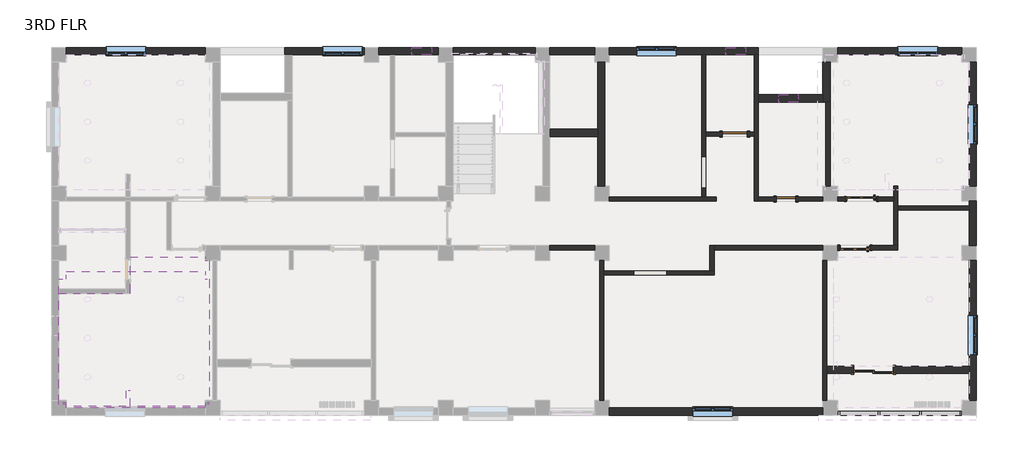
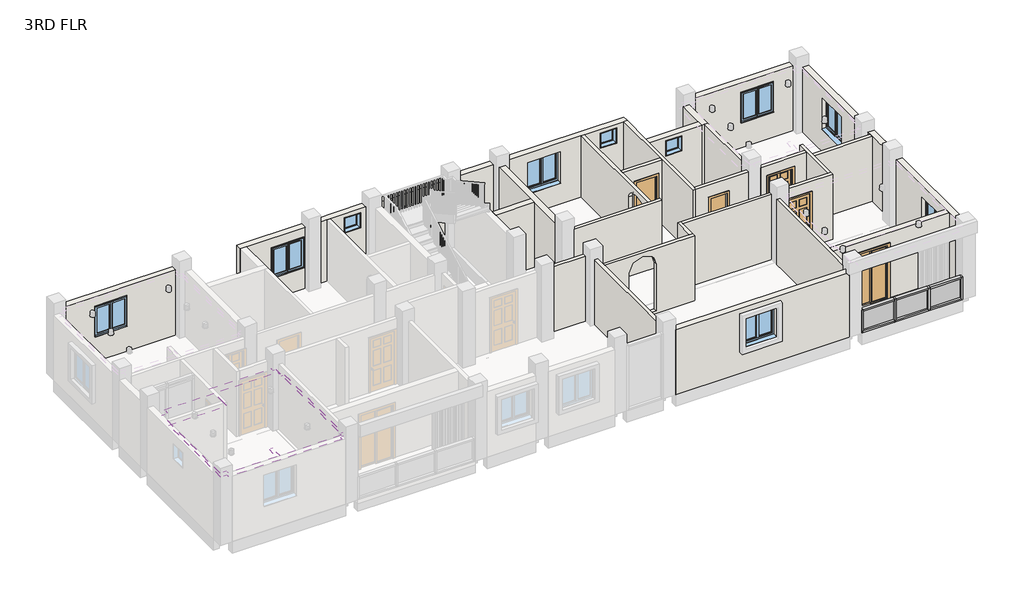
# One storey, part 2 of 5: 32 walls, 10 members, 10 windows, 5 doors, 3 plates, 2 coverings.
"""IFC4 building model written with IfcOpenShell, lengths in millimetres."""

from ifc_helpers import new_model, si_unit, point, frame, frame_2d, origin, place, context, project, spatial, polyline, circle_curve, ellipse_curve, trimmed, segment, composite_curve, outline, extrude, faceted_brep, transform, mapped, element, save
from ifc_brep_helpers import plane_surface, extruded_surface, advanced_brep
from components import door_double_sliding_4436dcad, door_c610b25b, door_03e3dfb5, single_flush_2_x_7_bath_room_door_025d1c86, door_1fe7f57d, member_5d96a33e, member_91edd790, member_410c6227, member_73c23c35, system_panel_glazed_2f542010, system_panel_glazed_876b4d55, window_80340324, w2_0001_4_x_4_window_9dec5fc7

model = new_model("IFC4")

# Units and contexts
model_context = context("Model", 3, world=origin())
ifc_project = project(units=[si_unit("LENGTHUNIT", "METRE", prefix="MILLI")], contexts=[model_context])

# Site, building, storey
site = spatial("IfcSite", under=ifc_project)
building = spatial("IfcBuilding", under=site)
storey = spatial("IfcBuildingStorey", under=building, Name="3RD FLR", Elevation=9448.8)

# Coverings
placement = place(None, origin())
element("IfcCovering", 1, ObjectType="GWB on Mtl. Stud", at=placement, inside=storey, context=model_context, shape_type="SweptSolid", body=[
    extrude(outline(polyline([(-15145.3456086, -10773.5679047), (-15145.3456086, -7363.1659448), (-12959.7401855, -7363.1659448), (-12959.7401855, -6244.0794704), (-10649.5456086, -6244.0794704), (-10649.5456086, -6358.3794704), (-10535.2456086, -6358.3794704), (-10535.2456086, -6963.5679047), (-10535.2456086, -10773.5679047), (-10649.5456086, -10773.5679047), (-10649.5456086, -10887.8679047), (-12959.7401855, -10887.8679047), (-14916.7456086, -10887.8679047), (-14916.7456086, -10773.5679047), (-15145.3456086, -10773.5679047)]), holes=[polyline([(-14840.5456086, -10583.0679047), (-10840.0456086, -10583.0679047), (-10840.0456086, -6548.8794704), (-12654.9401855, -6548.8794704), (-12654.9401855, -7667.9659448), (-14840.5456086, -7667.9659448), (-14840.5456086, -10583.0679047)])]), frame((0.0, 0.0, 11887.2), z_axis=(0.0, 0.0, 1.0), x_axis=(1.0, 0.0, 0.0)), (0.0, 0.0, 1.0), 107.95),
    extrude(outline(polyline([(-14688.1456086, -10430.6679047), (-14688.1456086, -7820.3659448), (-12502.5401855, -7820.3659448), (-12502.5401855, -6701.2794704), (-10992.4456086, -6701.2794704), (-10992.4456086, -10430.6679047), (-14688.1456086, -10430.6679047)]), holes=[polyline([(-14535.7456086, -7972.7659448), (-14535.7456086, -10278.2679047), (-11144.8456086, -10278.2679047), (-11144.8456086, -6853.6794704), (-12350.1401855, -6853.6794704), (-12350.1401855, -7972.7659448), (-14535.7456086, -7972.7659448)])]), frame((0.0, 0.0, 11887.2), z_axis=(0.0, 0.0, 1.0), x_axis=(1.0, 0.0, 0.0)), (0.0, 0.0, 1.0), 107.95),
])
element("IfcCovering", 2, ObjectType="GWB on Mtl. Stud", at=placement, inside=storey, context=model_context, shape_type="SweptSolid", body=[
    extrude(outline(polyline([(-14916.7456086, -6917.1794704), (-14916.7456086, -6688.5794704), (-10649.5456086, -6688.5794704), (-10649.5456086, -6917.1794704), (-10535.2456086, -6917.1794704), (-10535.2456086, -10727.1794704), (-10649.5456086, -10727.1794704), (-10649.5456086, -10841.4794704), (-12959.7401855, -10841.4794704), (-12959.7401855, -10360.3659448), (-13086.7401855, -10360.3659448), (-13086.7401855, -10841.4794704), (-14916.7456086, -10841.4794704), (-14916.7456086, -10727.1794704), (-15145.3456086, -10727.1794704), (-15145.3456086, -6917.1794704), (-14916.7456086, -6917.1794704)]), holes=[composite_curve([segment(trimmed(circle_curve(frame_2d((-14269.0456086, -7552.1794704)), 76.2), [point((-14345.2456086, -7552.1794704))], [point((-14192.8456086, -7552.1794704))], True, "CARTESIAN"), True, "CONTINUOUS"), segment(trimmed(circle_curve(frame_2d((-14269.0456086, -7552.1794704)), 76.2), [point((-14192.8456086, -7552.1794704))], [point((-14345.2456086, -7552.1794704))], True, "CARTESIAN"), True, "CONTINUOUS")], self_intersect=False), composite_curve([segment(trimmed(circle_curve(frame_2d((-14269.0456086, -9939.7794704)), 76.2), [point((-14345.2456086, -9939.7794704))], [point((-14192.8456086, -9939.7794704))], True, "CARTESIAN"), True, "CONTINUOUS"), segment(trimmed(circle_curve(frame_2d((-14269.0456086, -9939.7794704)), 76.2), [point((-14192.8456086, -9939.7794704))], [point((-14345.2456086, -9939.7794704))], True, "CARTESIAN"), True, "CONTINUOUS")], self_intersect=False), composite_curve([segment(trimmed(circle_curve(frame_2d((-14269.0456086, -8745.9794704)), 76.2), [point((-14345.2456086, -8745.9794704))], [point((-14192.8456086, -8745.9794704))], True, "CARTESIAN"), True, "CONTINUOUS"), segment(trimmed(circle_curve(frame_2d((-14269.0456086, -8745.9794704)), 76.2), [point((-14192.8456086, -8745.9794704))], [point((-14345.2456086, -8745.9794704))], True, "CARTESIAN"), True, "CONTINUOUS")], self_intersect=False), composite_curve([segment(trimmed(circle_curve(frame_2d((-11411.5456086, -7552.1794704)), 76.2), [point((-11335.3456086, -7552.1794704))], [point((-11487.7456086, -7552.1794704))], True, "CARTESIAN"), True, "CONTINUOUS"), segment(trimmed(circle_curve(frame_2d((-11411.5456086, -7552.1794704)), 76.2), [point((-11487.7456086, -7552.1794704))], [point((-11335.3456086, -7552.1794704))], True, "CARTESIAN"), True, "CONTINUOUS")], self_intersect=False), composite_curve([segment(trimmed(circle_curve(frame_2d((-11411.5456086, -9939.7794704)), 76.2), [point((-11335.3456086, -9939.7794704))], [point((-11487.7456086, -9939.7794704))], True, "CARTESIAN"), True, "CONTINUOUS"), segment(trimmed(circle_curve(frame_2d((-11411.5456086, -9939.7794704)), 76.2), [point((-11487.7456086, -9939.7794704))], [point((-11335.3456086, -9939.7794704))], True, "CARTESIAN"), True, "CONTINUOUS")], self_intersect=False)]), frame((0.0, 0.0, 12014.2), z_axis=(0.0, 0.0, 1.0), x_axis=(1.0, 0.0, 0.0)), (0.0, 0.0, 1.0), 107.95),
])

# Doors
door_double_sliding_shape = door_double_sliding_4436dcad(model_context)
element("IfcDoor", 3, ObjectType="Door-Double-Sliding", at=placement, inside=storey, context=model_context, shape_type="MappedRepresentation", body=[
    mapped(door_double_sliding_shape, transform((9879.3128058, -9592.4679047, 9448.8), x_axis=(-1.0, 0.0, 0.0), y_axis=(0.0, -1.0, 0.0), z_axis=(0.0, 0.0, 1.0))),
])
door_shape = door_c610b25b(model_context)
element("IfcDoor", 4, ObjectType="Door-Interior-Single-6_Panel-Wood : 36\" x 84\"", at=placement, inside=storey, context=model_context, shape_type="MappedRepresentation", body=[
    mapped(door_shape, transform((9511.0128058, -4462.9044704, 9448.8), x_axis=(-1.0, 0.0, 0.0), y_axis=(0.0, -1.0, 0.0), z_axis=(0.0, 0.0, 1.0))),
])
door_2_shape = door_03e3dfb5(model_context)
element("IfcDoor", 5, ObjectType="Door-Interior-Single-6_Panel-Wood : 36\" x 84\"", at=placement, inside=storey, context=model_context, shape_type="MappedRepresentation", body=[
    mapped(door_2_shape, transform((9307.8128058, -5967.8544704, 9448.8), x_axis=(-1.0, 0.0, 0.0), y_axis=(0.0, -1.0, 0.0), z_axis=(0.0, 0.0, 1.0))),
])
single_flush_2_x_7_bath_room_door_shape = single_flush_2_x_7_bath_room_door_025d1c86(model_context)
element("IfcDoor", 6, ObjectType="Single-Flush : 2' X 7' BATH ROOM DOOR", at=placement, inside=storey, context=model_context, shape_type="MappedRepresentation", body=[
    mapped(single_flush_2_x_7_bath_room_door_shape, transform((7190.4916602, -4466.0794704, 9448.8), x_axis=(1.0, 0.0, 0.0), y_axis=(0.0, 1.0, 0.0), z_axis=(0.0, 0.0, 1.0))),
])
door_3_shape = door_1fe7f57d(model_context)
element("IfcDoor", 7, ObjectType="Single-Flush : 30\" x 80\"", at=placement, inside=storey, context=model_context, shape_type="MappedRepresentation", body=[
    mapped(door_3_shape, transform((5615.6916602, -2472.1794704, 9448.8), x_axis=(1.0, 0.0, 0.0), y_axis=(0.0, 1.0, 0.0), z_axis=(0.0, 0.0, 1.0))),
])

# Members
member_shape = member_5d96a33e(model_context)
element("IfcMember", 8, ObjectType="Rectangular Mullion : 2.5\" x 5\" rectangular", at=placement, inside=storey, context=model_context, shape_type="MappedRepresentation", body=[
    mapped(member_shape, transform((12520.9128058, -11052.9679047, 10363.2), x_axis=(0.0, 0.0, 1.0), y_axis=(0.0, -1.0, 0.0), z_axis=(1.0, 0.0, 0.0))),
])
element("IfcMember", 9, ObjectType="Rectangular Mullion : 2.5\" x 5\" rectangular", at=placement, inside=storey, context=model_context, shape_type="MappedRepresentation", body=[
    mapped(member_shape, transform((10012.6628059, -11052.9679047, 10363.2), x_axis=(0.0, 0.0, 1.0), y_axis=(0.0, -1.0, 0.0), z_axis=(1.0, 0.0, 0.0))),
])
element("IfcMember", 10, ObjectType="Rectangular Mullion : 2.5\" x 5\" rectangular", at=placement, inside=storey, context=model_context, shape_type="MappedRepresentation", body=[
    mapped(member_shape, transform((8837.9128058, -11052.9679047, 9448.8), x_axis=(0.0, 0.0, -1.0), y_axis=(0.0, -1.0, 0.0), z_axis=(-1.0, 0.0, 0.0))),
])
element("IfcMember", 11, ObjectType="Rectangular Mullion : 2.5\" x 5\" rectangular", at=placement, inside=storey, context=model_context, shape_type="MappedRepresentation", body=[
    mapped(member_shape, transform((11346.1628057, -11052.9679047, 9448.8), x_axis=(0.0, 0.0, -1.0), y_axis=(0.0, -1.0, 0.0), z_axis=(-1.0, 0.0, 0.0))),
])
member_2_shape = member_91edd790(model_context)
element("IfcMember", 12, ObjectType="Rectangular Mullion : 2.5\" x 5\" rectangular", at=placement, inside=storey, context=model_context, shape_type="MappedRepresentation", body=[
    mapped(member_2_shape, transform((11282.6628057, -11052.9679047, 10363.2), x_axis=(0.0, 0.0, 1.0), y_axis=(0.0, -1.0, 0.0), z_axis=(1.0, 0.0, 0.0))),
])
element("IfcMember", 13, ObjectType="Rectangular Mullion : 2.5\" x 5\" rectangular", at=placement, inside=storey, context=model_context, shape_type="MappedRepresentation", body=[
    mapped(member_2_shape, transform((10076.1628059, -11052.9679047, 9448.8), x_axis=(0.0, 0.0, -1.0), y_axis=(0.0, -1.0, 0.0), z_axis=(-1.0, 0.0, 0.0))),
])
member_3_shape = member_410c6227(model_context)
element("IfcMember", 14, ObjectType="Rectangular Mullion : 2.5\" x 5\" rectangular", at=placement, inside=storey, context=model_context, shape_type="MappedRepresentation", body=[
    mapped(member_3_shape, transform((10044.4128059, -11052.9679047, 9448.8), x_axis=(1.0, 0.0, 0.0), y_axis=(0.0, -1.0, 0.0), z_axis=(0.0, 0.0, -1.0))),
])
element("IfcMember", 15, ObjectType="Rectangular Mullion : 2.5\" x 5\" rectangular", at=placement, inside=storey, context=model_context, shape_type="MappedRepresentation", body=[
    mapped(member_3_shape, transform((11314.4128057, -11052.9679047, 9448.8), x_axis=(1.0, 0.0, 0.0), y_axis=(0.0, -1.0, 0.0), z_axis=(0.0, 0.0, -1.0))),
])
member_4_shape = member_73c23c35(model_context)
element("IfcMember", 16, ObjectType="Rectangular Mullion : 2.5\" x 5\" rectangular", at=placement, inside=storey, context=model_context, shape_type="MappedRepresentation", body=[
    mapped(member_4_shape, transform((12584.4128058, -11052.9679047, 9448.8), x_axis=(1.0, 0.0, 0.0), y_axis=(0.0, -1.0, 0.0), z_axis=(0.0, 0.0, -1.0))),
])
element("IfcMember", 17, ObjectType="Rectangular Mullion : 2.5\" x 5\" rectangular", at=placement, inside=storey, context=model_context, shape_type="MappedRepresentation", body=[
    mapped(member_4_shape, transform((8774.4128058, -11052.9679047, 10363.2), x_axis=(-1.0, 0.0, 0.0), y_axis=(0.0, -1.0, 0.0), z_axis=(0.0, 0.0, 1.0))),
])

# Plates
system_panel_glazed_shape = system_panel_glazed_2f542010(model_context)
element("IfcPlate", 18, ObjectType="System Panel : Glazed", at=placement, inside=storey, context=model_context, shape_type="MappedRepresentation", body=[
    mapped(system_panel_glazed_shape, transform((9425.2878058, -11052.9679047, 9512.3), x_axis=(1.0, 0.0, 0.0), y_axis=(0.0, 1.0, 0.0), z_axis=(0.0, 0.0, 1.0))),
])
element("IfcPlate", 19, ObjectType="System Panel : Glazed", at=placement, inside=storey, context=model_context, shape_type="MappedRepresentation", body=[
    mapped(system_panel_glazed_shape, transform((11933.5378057, -11052.9679047, 9512.3), x_axis=(1.0, 0.0, 0.0), y_axis=(0.0, 1.0, 0.0), z_axis=(0.0, 0.0, 1.0))),
])
system_panel_glazed_2_shape = system_panel_glazed_876b4d55(model_context)
element("IfcPlate", 20, ObjectType="System Panel : Glazed", at=placement, inside=storey, context=model_context, shape_type="MappedRepresentation", body=[
    mapped(system_panel_glazed_2_shape, transform((10679.4128058, -11052.9679047, 9512.3), x_axis=(1.0, 0.0, 0.0), y_axis=(0.0, 1.0, 0.0), z_axis=(0.0, 0.0, 1.0))),
])

# Walls
element("IfcWall", 21, ObjectType="EXTERIOR WALL 9\"", at=placement, inside=storey, context=model_context, shape_type="SweptSolid", body=[
    extrude(outline(polyline([(9448.8, 1767.5916602), (9448.8, 8317.2128058), (12039.6, 8317.2128058), (12039.6, 1767.5916602), (9448.8, 1767.5916602)]), holes=[polyline([(10448.8, 5552.1916602), (10448.8, 4332.9916602), (11668.0, 4332.9916602), (11668.0, 5552.1916602), (10448.8, 5552.1916602)])]), frame((0.0, -11116.4679047, 0.0), z_axis=(0.0, 1.0, 0.0), x_axis=(0.0, 0.0, 1.0)), (0.0, 0.0, 1.0), 228.6),
])
element("IfcWall", 22, ObjectType="EXTERIOR WALL 9\"", at=placement, inside=storey, context=model_context, shape_type="Brep", body=[
    faceted_brep([(13041.6128058, -10659.2679047, 9448.8), (13041.6128058, -6358.3794704, 9448.8), (13041.6128058, -6358.3794704, 12039.6), (13041.6128058, -10659.2679047, 12039.6), (13041.6128058, -9262.2679047, 10363.2), (13041.6128058, -9262.2679047, 11582.4), (13041.6128058, -8043.0679047, 11582.4), (13041.6128058, -8043.0679047, 10363.2), (12813.0128058, -6358.3794704, 9448.8), (12813.0128058, -9605.1679047, 9448.8), (12813.0128058, -9833.7679047, 9448.8), (12813.0128058, -10659.2679047, 9448.8), (12813.0128058, -10659.2679047, 12039.6), (12813.0128058, -9833.7679047, 12039.6), (12813.0128058, -9605.1679047, 12039.6), (12813.0128058, -6358.3794704, 12039.6), (12813.0128058, -9262.2679047, 11582.4), (12813.0128058, -9262.2679047, 10363.2), (12813.0128058, -8043.0679047, 10363.2), (12813.0128058, -8043.0679047, 11582.4)], [[[0, 1, 2, 3], [4, 5, 6, 7]], [[8, 9, 10, 11, 12, 13, 14, 15], [16, 17, 18, 19]], [[1, 0, 11, 10, 9, 8]], [[2, 1, 8, 15]], [[3, 2, 15, 14, 13, 12]], [[0, 3, 12, 11]], [[5, 4, 17, 16]], [[6, 5, 16, 19]], [[7, 6, 19, 18]], [[4, 7, 18, 17]]]),
])
element("IfcWall", 23, ObjectType="EXTERIOR WALL 9\"", at=placement, inside=storey, context=model_context, shape_type="Brep", body=[
    faceted_brep([(13041.6128058, -5901.1794704, 9448.8), (13041.6128058, -4529.5794704, 9448.8), (13041.6128058, -4529.5794704, 12039.6), (13041.6128058, -5901.1794704, 12039.6), (12813.0128058, -5901.1794704, 9448.8), (12813.0128058, -5901.1794704, 12039.6), (12813.0128058, -4808.9794704, 12039.6), (12813.0128058, -4681.9794704, 12039.6), (12813.0128058, -4529.5794704, 12039.6), (12813.0128058, -4529.5794704, 9448.8), (12813.0128058, -4681.9794704, 9448.8), (12813.0128058, -4808.9794704, 9448.8)], [[[0, 1, 2, 3]], [[4, 5, 6, 7, 8, 9, 10, 11]], [[1, 0, 4, 11, 10, 9]], [[2, 1, 9, 8]], [[3, 2, 8, 7, 6, 5]], [[0, 3, 5, 4]]]),
])
element("IfcWall", 24, ObjectType="EXTERIOR WALL 9\"", at=placement, inside=storey, context=model_context, shape_type="SweptSolid", body=[
    extrude(outline(polyline([(-4072.3794704, 9448.8), (-4072.3794704, 12039.6), (-262.3794704, 12039.6), (-262.3794704, 9448.8), (-4072.3794704, 9448.8)]), holes=[polyline([(-2776.9794704, 10363.2), (-1557.7794704, 10363.2), (-1557.7794704, 11582.4), (-2776.9794704, 11582.4), (-2776.9794704, 10363.2)])]), frame((12813.0128058, 0.0, 0.0), z_axis=(1.0, 0.0, 0.0), x_axis=(0.0, 1.0, 0.0)), (0.0, 0.0, 1.0), 228.6),
])
element("IfcWall", 25, ObjectType="EXTERIOR WALL 9\"", at=placement, inside=storey, context=model_context, shape_type="SweptSolid", body=[
    extrude(outline(polyline([(9448.8, 12584.4128058), (12039.6, 12584.4128058), (12039.6, 8774.4128058), (9448.8, 8774.4128058), (9448.8, 12584.4128058)]), holes=[polyline([(10448.8, 10628.6128058), (11668.0, 10628.6128058), (11668.0, 11847.8128058), (10448.8, 11847.8128058), (10448.8, 10628.6128058)])]), frame((0.0, -33.7794704, 0.0), z_axis=(0.0, 1.0, 0.0), x_axis=(0.0, 0.0, 1.0)), (0.0, 0.0, 1.0), 228.6),
])
element("IfcWall", 26, ObjectType="EXTERIOR WALL 9\"", at=placement, inside=storey, context=model_context, shape_type="SweptSolid", body=[
    extrude(outline(polyline([(9448.8, -14916.7456086), (9448.8, -10649.5456086), (12039.6, -10649.5456086), (12039.6, -14916.7456086), (9448.8, -14916.7456086)]), holes=[polyline([(10448.8, -13697.5456086), (11668.0, -13697.5456086), (11668.0, -12478.3456086), (10448.8, -12478.3456086), (10448.8, -13697.5456086)])]), frame((0.0, -33.7794704, 0.0), z_axis=(0.0, 1.0, 0.0), x_axis=(0.0, 0.0, 1.0)), (0.0, 0.0, 1.0), 228.6),
])
element("IfcWall", 27, ObjectType="EXTERIOR WALL 9\"", at=placement, inside=storey, context=model_context, shape_type="SweptSolid", body=[
    extrude(outline(polyline([(9448.8, 8444.2128058), (9448.8, 9269.7128058), (11582.4, 9269.7128058), (11582.4, 10488.9128058), (9448.8, 10488.9128058), (9448.8, 12813.0128058), (12039.6, 12813.0128058), (12039.6, 8444.2128058), (9448.8, 8444.2128058)])), frame((0.0, -9833.7679047, 0.0), z_axis=(0.0, 1.0, 0.0), x_axis=(0.0, 0.0, 1.0)), (0.0, 0.0, 1.0), 228.6),
])
element("IfcWall", 28, ObjectType="EXTERIOR WALL 9\"", at=placement, inside=storey, context=model_context, shape_type="Brep", body=[
    faceted_brep([(-5772.7456086, 194.8205296, 9448.8), (-8211.1456086, 194.8205296, 9448.8), (-8211.1456086, 194.8205296, 12039.6), (-5772.7456086, 194.8205296, 12039.6), (-7042.7456086, 194.8205296, 10448.8), (-5823.5456086, 194.8205296, 10448.8), (-5823.5456086, 194.8205296, 11668.0), (-7042.7456086, 194.8205296, 11668.0), (-5772.7456086, -33.7794704, 9448.8), (-5772.7456086, -33.7794704, 12039.6), (-7982.5456086, -33.7794704, 12039.6), (-8211.1456086, -33.7794704, 12039.6), (-8211.1456086, -33.7794704, 9448.8), (-7982.5456086, -33.7794704, 9448.8), (-7042.7456086, -33.7794704, 10448.8), (-7042.7456086, -33.7794704, 11668.0), (-5823.5456086, -33.7794704, 11668.0), (-5823.5456086, -33.7794704, 10448.8)], [[[0, 1, 2, 3], [4, 5, 6, 7]], [[8, 9, 10, 11, 12, 13], [14, 15, 16, 17]], [[1, 0, 8, 13, 12]], [[3, 2, 11, 10, 9]], [[0, 3, 9, 8]], [[2, 1, 12, 11]], [[15, 14, 4, 7]], [[16, 15, 7, 6]], [[17, 16, 6, 5]], [[14, 17, 5, 4]]]),
])
element("IfcWall", 29, ObjectType="EXTERIOR WALL 9\"", at=placement, inside=storey, context=model_context, shape_type="Brep", body=[
    faceted_brep([(-5315.5456086, -33.7794704, 9448.8), (-4959.9456086, -33.7794704, 9448.8), (-4832.9456086, -33.7794704, 9448.8), (-3486.7456086, -33.7794704, 9448.8), (-3486.7456086, -33.7794704, 12039.6), (-4832.9456086, -33.7794704, 12039.6), (-4959.9456086, -33.7794704, 12039.6), (-5315.5456086, -33.7794704, 12039.6), (-3689.9456086, -33.7794704, 11887.2), (-3689.9456086, -33.7794704, 11277.6), (-4299.5456086, -33.7794704, 11277.6), (-4299.5456086, -33.7794704, 11887.2), (-3486.7456086, 194.8205296, 9448.8), (-5315.5456086, 194.8205296, 9448.8), (-5315.5456086, 194.8205296, 12039.6), (-3486.7456086, 194.8205296, 12039.6), (-3689.9456086, 194.8205296, 11277.6), (-3689.9456086, 194.8205296, 11887.2), (-4299.5456086, 194.8205296, 11887.2), (-4299.5456086, 194.8205296, 11277.6)], [[[0, 1, 2, 3, 4, 5, 6, 7], [8, 9, 10, 11]], [[12, 13, 14, 15], [16, 17, 18, 19]], [[3, 2, 1, 0, 13, 12]], [[4, 3, 12, 15]], [[7, 6, 5, 4, 15, 14]], [[0, 7, 14, 13]], [[8, 17, 16, 9]], [[9, 16, 19, 10]], [[10, 19, 18, 11]], [[17, 8, 11, 18]]]),
])
element("IfcWall", 30, ObjectType="EXTERIOR WALL 9\"", at=placement, inside=storey, context=model_context, shape_type="SweptSolid", body=[
    extrude(outline(polyline([(-518.4083398, -33.7794704), (-3029.5456086, -33.7794704), (-3029.5456086, 194.8205296), (-518.4083398, 194.8205296), (-518.4083398, -33.7794704)])), frame((0.0, 0.0, 9448.8), z_axis=(0.0, 0.0, 1.0), x_axis=(1.0, 0.0, 0.0)), (0.0, 0.0, 1.0), 2590.8),
])
element("IfcWall", 31, ObjectType="EXTERIOR WALL 9\"", at=placement, inside=storey, context=model_context, shape_type="SweptSolid", body=[
    extrude(outline(polyline([(1310.3916602, -33.7794704), (-61.2083398, -33.7794704), (-61.2083398, 194.8205296), (1310.3916602, 194.8205296), (1310.3916602, -33.7794704)])), frame((0.0, 0.0, 9448.8), z_axis=(0.0, 0.0, 1.0), x_axis=(1.0, 0.0, 0.0)), (0.0, 0.0, 1.0), 2590.8),
])
element("IfcWall", 32, ObjectType="EXTERIOR WALL 9\"", at=placement, inside=storey, context=model_context, shape_type="Brep", body=[
    faceted_brep([(1767.5916602, -33.7794704, 9448.8), (4599.6916602, -33.7794704, 9448.8), (4726.6916602, -33.7794704, 9448.8), (6212.5916602, -33.7794704, 9448.8), (6339.5916602, -33.7794704, 9448.8), (6339.5916602, -33.7794704, 12039.6), (6212.5916602, -33.7794704, 12039.6), (4726.6916602, -33.7794704, 12039.6), (4599.6916602, -33.7794704, 12039.6), (1767.5916602, -33.7794704, 12039.6), (3824.9916602, -33.7794704, 11668.0), (3824.9916602, -33.7794704, 10448.8), (2605.7916602, -33.7794704, 10448.8), (2605.7916602, -33.7794704, 11668.0), (5945.8916602, -33.7794704, 11887.2), (5945.8916602, -33.7794704, 11277.6), (5336.2916602, -33.7794704, 11277.6), (5336.2916602, -33.7794704, 11887.2), (6339.5916602, 194.8205296, 9448.8), (1767.5916602, 194.8205296, 9448.8), (1767.5916602, 194.8205296, 12039.6), (6339.5916602, 194.8205296, 12039.6), (3824.9916602, 194.8205296, 10448.8), (3824.9916602, 194.8205296, 11668.0), (2605.7916602, 194.8205296, 11668.0), (2605.7916602, 194.8205296, 10448.8), (5945.8916602, 194.8205296, 11277.6), (5945.8916602, 194.8205296, 11887.2), (5336.2916602, 194.8205296, 11887.2), (5336.2916602, 194.8205296, 11277.6)], [[[0, 1, 2, 3, 4, 5, 6, 7, 8, 9], [10, 11, 12, 13], [14, 15, 16, 17]], [[18, 19, 20, 21], [22, 23, 24, 25], [26, 27, 28, 29]], [[4, 3, 2, 1, 0, 19, 18]], [[9, 8, 7, 6, 5, 21, 20]], [[0, 9, 20, 19]], [[5, 4, 18, 21]], [[23, 22, 11, 10]], [[24, 23, 10, 13]], [[25, 24, 13, 12]], [[22, 25, 12, 11]], [[14, 27, 26, 15]], [[15, 26, 29, 16]], [[16, 29, 28, 17]], [[27, 14, 17, 28]]]),
])
element("IfcWall", 33, ObjectType="EXTERIOR WALL 9\"", at=placement, inside=storey, context=model_context, shape_type="Brep", body=[
    faceted_brep([(8317.2128058, -262.3794704, 9448.8), (8317.2128058, -1252.9794704, 9448.8), (8317.2128058, -1481.5794704, 9448.8), (8317.2128058, -1481.5794704, 12039.6), (8317.2128058, -1252.9794704, 12039.6), (8317.2128058, -262.3794704, 12039.6), (8545.8128058, -262.3794704, 9448.8), (8545.8128058, -262.3794704, 12039.6), (8545.8128058, -1481.5794704, 12039.6), (8545.8128058, -1481.5794704, 9448.8), (8418.8128058, -1481.5794704, 9448.8), (8418.8128058, -1481.5794704, 12039.6)], [[[0, 1, 2, 3, 4, 5]], [[6, 7, 8, 9]], [[2, 1, 0, 6, 9, 10]], [[5, 4, 3, 11, 8, 7]], [[0, 5, 7, 6]], [[3, 2, 10, 9, 8, 11]]]),
])
element("IfcWall", 34, ObjectType="EXTERIOR WALL 9\"", at=placement, inside=storey, context=model_context, shape_type="SweptSolid", body=[
    extrude(outline(polyline([(9448.8, 6339.5916602), (9448.8, 8317.2128058), (12039.6, 8317.2128058), (12039.6, 6339.5916602), (9448.8, 6339.5916602)]), holes=[polyline([(11887.2, 7571.4916602), (11277.6, 7571.4916602), (11277.6, 6961.8916602), (11887.2, 6961.8916602), (11887.2, 7571.4916602)])]), frame((0.0, -1481.5794704, 0.0), z_axis=(0.0, 1.0, 0.0), x_axis=(0.0, 0.0, 1.0)), (0.0, 0.0, 1.0), 228.6),
])
element("IfcWall", 35, ObjectType="EXTERIOR WALL 9\"", at=placement, inside=storey, context=model_context, shape_type="Brep", body=[
    faceted_brep([(1399.2916602, -262.3794704, 9448.8), (1399.2916602, -2319.7794704, 9448.8), (1399.2916602, -2548.3794704, 9448.8), (1399.2916602, -4072.3794704, 9448.8), (1399.2916602, -4072.3794704, 12039.6), (1399.2916602, -2548.3794704, 12039.6), (1399.2916602, -2319.7794704, 12039.6), (1399.2916602, -262.3794704, 12039.6), (1627.8916602, -262.3794704, 9448.8), (1627.8916602, -262.3794704, 12039.6), (1627.8916602, -4072.3794704, 12039.6), (1627.8916602, -4072.3794704, 9448.8)], [[[0, 1, 2, 3, 4, 5, 6, 7]], [[8, 9, 10, 11]], [[3, 2, 1, 0, 8, 11]], [[4, 3, 11, 10]], [[7, 6, 5, 4, 10, 9]], [[0, 7, 9, 8]]]),
])
element("IfcWall", 36, ObjectType="EXTERIOR WALL 9\"", at=placement, inside=storey, context=model_context, shape_type="SweptSolid", body=[
    extrude(outline(polyline([(1399.2916602, -2548.3794704), (-61.2083398, -2548.3794704), (-61.2083398, -2319.7794704), (1399.2916602, -2319.7794704), (1399.2916602, -2548.3794704)])), frame((0.0, 0.0, 9448.8), z_axis=(0.0, 0.0, 1.0), x_axis=(1.0, 0.0, 0.0)), (0.0, 0.0, 1.0), 2590.8),
])
element("IfcWall", 37, ObjectType="INTERIOR WALL 5\"", at=placement, inside=storey, context=model_context, shape_type="Brep", body=[
    faceted_brep([(1589.7916602, -10659.2679047, 9448.8), (1589.7916602, -6802.8794704, 9448.8), (1589.7916602, -6675.8794704, 9448.8), (1589.7916602, -6358.3794704, 9448.8), (1589.7916602, -6358.3794704, 12039.6), (1589.7916602, -6675.8794704, 12039.6), (1589.7916602, -6802.8794704, 12039.6), (1589.7916602, -10659.2679047, 12039.6), (1462.7916602, -10659.2679047, 9448.8), (1462.7916602, -10659.2679047, 12039.6), (1462.7916602, -6358.3794704, 12039.6), (1462.7916602, -6358.3794704, 9448.8)], [[[0, 1, 2, 3, 4, 5, 6, 7]], [[8, 9, 10, 11]], [[3, 2, 1, 0, 8, 11]], [[4, 3, 11, 10]], [[7, 6, 5, 4, 10, 9]], [[0, 7, 9, 8]]]),
])
element("IfcWall", 38, ObjectType="INTERIOR WALL 5\"", at=placement, inside=storey, context=model_context, shape_type="Brep", body=[
    faceted_brep([(8444.2128058, -10659.2679047, 9448.8), (8444.2128058, -9833.7679047, 9448.8), (8444.2128058, -9605.1679047, 9448.8), (8444.2128058, -6358.3794704, 9448.8), (8444.2128058, -6358.3794704, 12039.6), (8444.2128058, -9605.1679047, 12039.6), (8444.2128058, -9833.7679047, 12039.6), (8444.2128058, -10659.2679047, 12039.6), (8317.2128058, -10659.2679047, 9448.8), (8317.2128058, -10659.2679047, 12039.6), (8317.2128058, -6358.3794704, 12039.6), (8317.2128058, -6358.3794704, 9448.8)], [[[0, 1, 2, 3, 4, 5, 6, 7]], [[8, 9, 10, 11]], [[3, 2, 1, 0, 8, 11]], [[4, 3, 11, 10]], [[7, 6, 5, 4, 10, 9]], [[0, 7, 9, 8]]]),
])
element("IfcWall", 39, ObjectType="INTERIOR WALL 5\"", at=placement, inside=storey, context=model_context, shape_type="SweptSolid", body=[
    extrude(outline(polyline([(10628.6128058, -4681.9794704), (12813.0128058, -4681.9794704), (12813.0128058, -4808.9794704), (10628.6128058, -4808.9794704), (10628.6128058, -4681.9794704)])), frame((0.0, 0.0, 9448.8), z_axis=(0.0, 0.0, 1.0), x_axis=(1.0, 0.0, 0.0)), (0.0, 0.0, 1.0), 2590.8),
])
element("IfcWall", 40, ObjectType="INTERIOR WALL 5\"", at=placement, inside=storey, context=model_context, shape_type="Brep", body=[
    faceted_brep([(10628.6128058, -6028.1794704, 12039.6), (8774.4128058, -6028.1794704, 12039.6), (8774.4128058, -6028.1794704, 9448.8), (8825.2128058, -6028.1794704, 9448.8), (8825.2128058, -6028.1794704, 11607.8), (9790.4128058, -6028.1794704, 11607.8), (9790.4128058, -6028.1794704, 9448.8), (10628.6128058, -6028.1794704, 9448.8), (8774.4128058, -5901.1794704, 12039.6), (10501.6128058, -5901.1794704, 12039.6), (10628.6128058, -5901.1794704, 12039.6), (10628.6128058, -5901.1794704, 9448.8), (10501.6128058, -5901.1794704, 9448.8), (9790.4128058, -5901.1794704, 9448.8), (9790.4128058, -5901.1794704, 11607.8), (8825.2128058, -5901.1794704, 11607.8), (8825.2128058, -5901.1794704, 9448.8), (8774.4128058, -5901.1794704, 9448.8)], [[[0, 1, 2, 3, 4, 5, 6, 7]], [[8, 9, 10, 11, 12, 13, 14, 15, 16, 17]], [[2, 17, 16, 3]], [[11, 7, 6, 13, 12]], [[1, 0, 10, 9, 8]], [[2, 1, 8, 17]], [[0, 7, 11, 10]], [[15, 4, 3, 16]], [[4, 15, 14, 5]], [[5, 14, 13, 6]]]),
])
element("IfcWall", 41, ObjectType="INTERIOR WALL 5\"", at=placement, inside=storey, context=model_context, shape_type="Brep", body=[
    faceted_brep([(10628.6128058, -5901.1794704, 9448.8), (10628.6128058, -4808.9794704, 9448.8), (10628.6128058, -4681.9794704, 9448.8), (10628.6128058, -4072.3794704, 9448.8), (10628.6128058, -4072.3794704, 12039.6), (10628.6128058, -4681.9794704, 12039.6), (10628.6128058, -4808.9794704, 12039.6), (10628.6128058, -5901.1794704, 12039.6), (10501.6128058, -5901.1794704, 9448.8), (10501.6128058, -5901.1794704, 12039.6), (10501.6128058, -4529.5794704, 12039.6), (10501.6128058, -4402.5794704, 12039.6), (10501.6128058, -4072.3794704, 12039.6), (10501.6128058, -4072.3794704, 9448.8), (10501.6128058, -4402.5794704, 9448.8), (10501.6128058, -4529.5794704, 9448.8)], [[[0, 1, 2, 3, 4, 5, 6, 7]], [[8, 9, 10, 11, 12, 13, 14, 15]], [[3, 2, 1, 0, 8, 15, 14, 13]], [[4, 3, 13, 12]], [[7, 6, 5, 4, 12, 11, 10, 9]], [[0, 7, 9, 8]]]),
])
element("IfcWall", 42, ObjectType="INTERIOR WALL 5\"", at=placement, inside=storey, context=model_context, shape_type="Brep", body=[
    faceted_brep([(6212.5916602, -33.7794704, 9448.8), (6212.5916602, -2408.6794704, 9448.8), (6212.5916602, -2535.6794704, 9448.8), (6212.5916602, -4529.5794704, 9448.8), (6212.5916602, -4529.5794704, 12039.6), (6212.5916602, -2535.6794704, 12039.6), (6212.5916602, -2408.6794704, 12039.6), (6212.5916602, -33.7794704, 12039.6), (6339.5916602, -33.7794704, 9448.8), (6339.5916602, -33.7794704, 12039.6), (6339.5916602, -1252.9794704, 12039.6), (6339.5916602, -1481.5794704, 12039.6), (6339.5916602, -4402.5794704, 12039.6), (6339.5916602, -4529.5794704, 12039.6), (6339.5916602, -4529.5794704, 9448.8), (6339.5916602, -4402.5794704, 9448.8), (6339.5916602, -1481.5794704, 9448.8), (6339.5916602, -1252.9794704, 9448.8)], [[[0, 1, 2, 3, 4, 5, 6, 7]], [[8, 9, 10, 11, 12, 13, 14, 15, 16, 17]], [[3, 2, 1, 0, 8, 17, 16, 15, 14]], [[7, 6, 5, 4, 13, 12, 11, 10, 9]], [[0, 7, 9, 8]], [[4, 3, 14, 13]]]),
])
element("IfcWall", 43, ObjectType="INTERIOR WALL 5\"", at=placement, inside=storey, context=model_context, shape_type="SweptSolid", body=[
    extrude(outline(polyline([(8418.8128058, -4072.3794704), (8418.8128058, -1481.5794704), (8545.8128058, -1481.5794704), (8545.8128058, -4072.3794704), (8418.8128058, -4072.3794704)])), frame((0.0, 0.0, 9448.8), z_axis=(0.0, 0.0, 1.0), x_axis=(1.0, 0.0, 0.0)), (0.0, 0.0, 1.0), 2590.8),
])
element("IfcWall", 44, ObjectType="INTERIOR WALL 5\"", at=placement, inside=storey, context=model_context, shape_type="Brep", body=[
    faceted_brep([(1767.5916602, -4529.5794704, 9448.8), (5044.1916602, -4529.5794704, 9448.8), (5044.1916602, -4529.5794704, 12039.6), (1767.5916602, -4529.5794704, 12039.6), (1767.5916602, -4402.5794704, 9448.8), (1767.5916602, -4402.5794704, 12039.6), (4599.6916602, -4402.5794704, 12039.6), (4726.6916602, -4402.5794704, 12039.6), (5044.1916602, -4402.5794704, 12039.6), (5044.1916602, -4402.5794704, 9448.8), (4726.6916602, -4402.5794704, 9448.8), (4599.6916602, -4402.5794704, 9448.8)], [[[0, 1, 2, 3]], [[4, 5, 6, 7, 8, 9, 10, 11]], [[1, 0, 4, 11, 10, 9]], [[2, 1, 9, 8]], [[3, 2, 8, 7, 6, 5]], [[0, 3, 5, 4]]]),
])
element("IfcWall", 45, ObjectType="INTERIOR WALL 5\"", at=placement, inside=storey, context=model_context, shape_type="AdvancedBrep", body=[
    advanced_brep(
    [(4599.6916602, -33.7794704, 9448.8), (4599.6916602, -4402.5794704, 9448.8), (4599.6916602, -4402.5794704, 12039.6), (4599.6916602, -33.7794704, 12039.6), (4599.6916602, -3162.9760679, 11507.4701015), (4599.6916602, -4128.1760679, 11507.4701015), (4599.6916602, -4128.1760679, 9627.8701015), (4599.6916602, -3162.9760679, 9627.8701015), (4726.6916602, -33.7794704, 9448.8), (4726.6916602, -33.7794704, 12039.6), (4726.6916602, -2408.6794704, 12039.6), (4726.6916602, -2535.6794704, 12039.6), (4726.6916602, -4402.5794704, 12039.6), (4726.6916602, -4402.5794704, 9448.8), (4726.6916602, -2535.6794704, 9448.8), (4726.6916602, -2408.6794704, 9448.8), (4726.6916602, -3162.9760679, 11507.4701015), (4726.6916602, -3162.9760679, 9627.8701015), (4726.6916602, -4128.1760679, 9627.8701015), (4726.6916602, -4128.1760679, 11507.4701015)],
    [
        (0, 1),
        (1, 2),
        (2, 3),
        (3, 0),
        (4, 5, ellipse_curve(frame((4599.6916602, -3645.5760679, 11507.4701015), z_axis=(1.0, 0.0, 0.0), x_axis=(0.0, -1.0, 0.0)), 482.6, 330.2)),
        (5, 6),
        (6, 7),
        (7, 4),
        (8, 9),
        (9, 10),
        (10, 11),
        (11, 12),
        (12, 13),
        (13, 14),
        (14, 15),
        (15, 8),
        (16, 17),
        (17, 18),
        (18, 19),
        (19, 16, ellipse_curve(frame((4726.6916602, -3645.5760679, 11507.4701015), z_axis=(-1.0, 0.0, 0.0), x_axis=(0.0, -1.0, 0.0)), 482.6, 330.2)),
        (3, 9),
        (8, 0),
        (1, 13),
        (12, 2),
        (4, 16),
        (19, 5),
        (18, 6),
        (17, 7),
    ],
    [
        plane_surface(frame((4599.6916602, 80.5205296, 9448.8), z_axis=(-1.0, 0.0, 0.0), x_axis=(0.0, -1.0, 0.0))),
        plane_surface(frame((4726.6916602, 80.5205296, 9448.8), z_axis=(1.0, 0.0, 0.0), x_axis=(0.0, 1.0, 0.0))),
        plane_surface(frame((1784.6412895, -33.7794704, 9448.8), z_axis=(0.0, 1.0, 0.0), x_axis=(1.0, 0.0, 0.0))),
        plane_surface(frame((1767.5916602, -4402.5794704, 9448.8), z_axis=(0.0, -1.0, 0.0), x_axis=(-1.0, 0.0, 0.0))),
        plane_surface(frame((4599.6916602, 80.5205296, 9448.8), z_axis=(0.0, 0.0, -1.0), x_axis=(1.0, 0.0, 0.0))),
        plane_surface(frame((4599.6916602, -4466.0794704, 12039.6), z_axis=(0.0, 0.0, 1.0), x_axis=(1.0, 0.0, 0.0))),
        extruded_surface(trimmed(ellipse_curve(frame((4790.1916602, -3645.5760679, 11507.4701015), z_axis=(1.0, 0.0, 0.0), x_axis=(0.0, -1.0, 0.0)), 482.6, 330.2), [point((4790.1916602, -3162.9760679, 11507.4701015))], [point((4790.1916602, -4128.1760679, 11507.4701015))], True, "CARTESIAN"), (-127.0, 0.0, 0.0), 127.0),
        plane_surface(frame((4599.6916602, -4128.1760679, 11507.4701015), z_axis=(0.0, 1.0, 0.0), x_axis=(1.0, 0.0, 0.0))),
        plane_surface(frame((4599.6916602, -4128.1760679, 9627.8701015), z_axis=(0.0, 0.0, 1.0), x_axis=(1.0, 0.0, 0.0))),
        plane_surface(frame((4599.6916602, -3162.9760679, 9627.8701015), z_axis=(0.0, -1.0, 0.0), x_axis=(1.0, 0.0, 0.0))),
    ],
    [
        (0, [[1, 2, 3, 4], [5, 6, 7, 8]]),
        (1, [[9, 10, 11, 12, 13, 14, 15, 16], [17, 18, 19, 20]]),
        (2, [[-4, 21, -9, 22]]),
        (3, [[-2, 23, -13, 24]]),
        (4, [[-1, -22, -16, -15, -14, -23]]),
        (5, [[-3, -24, -12, -11, -10, -21]]),
        (6, [[-5, 25, -20, 26]]),
        (7, [[-6, -26, -19, 27]]),
        (8, [[-7, -27, -18, 28]]),
        (9, [[-8, -28, -17, -25]]),
    ],
),
])
element("IfcWall", 46, ObjectType="INTERIOR WALL 5\"", at=placement, inside=storey, context=model_context, shape_type="SweptSolid", body=[
    extrude(outline(polyline([(11480.8, 5996.6916602), (9448.8, 5996.6916602), (9448.8, 6212.5916602), (12039.6, 6212.5916602), (12039.6, 4726.6916602), (9448.8, 4726.6916602), (9448.8, 5234.6916602), (11480.8, 5234.6916602), (11480.8, 5996.6916602)])), frame((0.0, -2535.6794704, 0.0), z_axis=(0.0, 1.0, 0.0), x_axis=(0.0, 0.0, 1.0)), (0.0, 0.0, 1.0), 127.0),
])
element("IfcWall", 47, ObjectType="INTERIOR WALL 5\"", at=placement, inside=storey, context=model_context, shape_type="SweptSolid", body=[
    extrude(outline(polyline([(11480.8, 7495.2916602), (9448.8, 7495.2916602), (9448.8, 8317.2128058), (12039.6, 8317.2128058), (12039.6, 6339.5916602), (9448.8, 6339.5916602), (9448.8, 6885.6916602), (11480.8, 6885.6916602), (11480.8, 7495.2916602)])), frame((0.0, -4529.5794704, 0.0), z_axis=(0.0, 1.0, 0.0), x_axis=(0.0, 0.0, 1.0)), (0.0, 0.0, 1.0), 127.0),
])
element("IfcWall", 48, ObjectType="INTERIOR WALL 5\"", at=placement, inside=storey, context=model_context, shape_type="SweptSolid", body=[
    extrude(outline(polyline([(12039.6, 10501.6128058), (12039.6, 8774.4128058), (9448.8, 8774.4128058), (9448.8, 9028.4128058), (11607.8, 9028.4128058), (11607.8, 9993.6128058), (9448.8, 9993.6128058), (9448.8, 10501.6128058), (12039.6, 10501.6128058)])), frame((0.0, -4529.5794704, 0.0), z_axis=(0.0, 1.0, 0.0), x_axis=(0.0, 0.0, 1.0)), (0.0, 0.0, 1.0), 127.0),
])
element("IfcWall", 49, ObjectType="INTERIOR WALL 5\"", at=placement, inside=storey, context=model_context, shape_type="SweptSolid", body=[
    extrude(outline(polyline([(-61.2083398, -5901.1794704), (1310.3916602, -5901.1794704), (1310.3916602, -6028.1794704), (-61.2083398, -6028.1794704), (-61.2083398, -5901.1794704)])), frame((0.0, 0.0, 9448.8), z_axis=(0.0, 0.0, 1.0), x_axis=(1.0, 0.0, 0.0)), (0.0, 0.0, 1.0), 2590.8),
])
element("IfcWall", 50, ObjectType="INTERIOR WALL 5\"", at=placement, inside=storey, context=model_context, shape_type="AdvancedBrep", body=[
    advanced_brep(
    [(1589.7916602, -6802.8794704, 9448.8), (4980.6916602, -6802.8794704, 9448.8), (4980.6916602, -6802.8794704, 12039.6), (1589.7916602, -6802.8794704, 12039.6), (2514.6258025, -6802.8794704, 11411.5597277), (3530.6258025, -6802.8794704, 11411.5597277), (3530.6258025, -6802.8794704, 9557.3597277), (2514.6258025, -6802.8794704, 9557.3597277), (1589.7916602, -6675.8794704, 9448.8), (1589.7916602, -6675.8794704, 12039.6), (4853.6916602, -6675.8794704, 12039.6), (4980.6916602, -6675.8794704, 12039.6), (4980.6916602, -6675.8794704, 9448.8), (4853.6916602, -6675.8794704, 9448.8), (2514.6258025, -6675.8794704, 11411.5597277), (2514.6258025, -6675.8794704, 9557.3597277), (3530.6258025, -6675.8794704, 9557.3597277), (3530.6258025, -6675.8794704, 11411.5597277)],
    [
        (0, 1),
        (1, 2),
        (2, 3),
        (3, 0),
        (4, 5, ellipse_curve(frame((3022.6258025, -6802.8794704, 11411.5597277), z_axis=(0.0, 1.0, 0.0), x_axis=(-1.0, 0.0, 0.0)), 508.0, 482.6)),
        (5, 6),
        (6, 7),
        (7, 4),
        (8, 9),
        (9, 10),
        (10, 11),
        (11, 12),
        (12, 13),
        (13, 8),
        (14, 15),
        (15, 16),
        (16, 17),
        (17, 14, ellipse_curve(frame((3022.6258025, -6675.8794704, 11411.5597277), z_axis=(0.0, -1.0, 0.0), x_axis=(-1.0, 0.0, 0.0)), 508.0, 482.6)),
        (3, 9),
        (8, 0),
        (1, 12),
        (11, 2),
        (4, 14),
        (17, 5),
        (16, 6),
        (15, 7),
    ],
    [
        plane_surface(frame((1526.2916602, -6802.8794704, 9448.8), z_axis=(0.0, -1.0, 0.0), x_axis=(1.0, 0.0, 0.0))),
        plane_surface(frame((1526.2916602, -6675.8794704, 9448.8), z_axis=(0.0, 1.0, 0.0), x_axis=(-1.0, 0.0, 0.0))),
        plane_surface(frame((1589.7916602, -10648.7570633, 9448.8), z_axis=(-1.0, 0.0, 0.0), x_axis=(0.0, 1.0, 0.0))),
        plane_surface(frame((4980.6916602, -6675.8794704, 9448.8), z_axis=(1.0, 0.0, 0.0), x_axis=(0.0, 1.0, 0.0))),
        plane_surface(frame((1526.2916602, -6802.8794704, 9448.8), z_axis=(0.0, 0.0, -1.0), x_axis=(0.0, 1.0, 0.0))),
        plane_surface(frame((4917.1916602, -6802.8794704, 12039.6), z_axis=(0.0, 0.0, 1.0), x_axis=(0.0, 1.0, 0.0))),
        extruded_surface(trimmed(ellipse_curve(frame((3022.6258025, -6612.3794704, 11411.5597277), z_axis=(0.0, 1.0, 0.0), x_axis=(-1.0, 0.0, 0.0)), 508.0, 482.6), [point((2514.6258025, -6612.3794704, 11411.5597277))], [point((3530.6258025, -6612.3794704, 11411.5597277))], True, "CARTESIAN"), (0.0, -127.0, 0.0), 127.0),
        plane_surface(frame((3530.6258025, -6802.8794704, 11411.5597277), z_axis=(-1.0, 0.0, 0.0), x_axis=(0.0, 1.0, 0.0))),
        plane_surface(frame((3530.6258025, -6802.8794704, 9557.3597277), z_axis=(0.0, 0.0, 1.0), x_axis=(0.0, 1.0, 0.0))),
        plane_surface(frame((2514.6258025, -6802.8794704, 9557.3597277), z_axis=(1.0, 0.0, 0.0), x_axis=(0.0, 1.0, 0.0))),
    ],
    [
        (0, [[1, 2, 3, 4], [5, 6, 7, 8]]),
        (1, [[9, 10, 11, 12, 13, 14], [15, 16, 17, 18]]),
        (2, [[-4, 19, -9, 20]]),
        (3, [[-2, 21, -12, 22]]),
        (4, [[-1, -20, -14, -13, -21]]),
        (5, [[-3, -22, -11, -10, -19]]),
        (6, [[-5, 23, -18, 24]]),
        (7, [[-6, -24, -17, 25]]),
        (8, [[-7, -25, -16, 26]]),
        (9, [[-8, -26, -15, -23]]),
    ],
),
])
element("IfcWall", 51, ObjectType="INTERIOR WALL 5\"", at=placement, inside=storey, context=model_context, shape_type="Brep", body=[
    faceted_brep([(4980.6916602, -6675.8794704, 9448.8), (4980.6916602, -6028.1794704, 9448.8), (4980.6916602, -5901.1794704, 9448.8), (4980.6916602, -5901.1794704, 12039.6), (4980.6916602, -6028.1794704, 12039.6), (4980.6916602, -6675.8794704, 12039.6), (4853.6916602, -6675.8794704, 9448.8), (4853.6916602, -6675.8794704, 12039.6), (4853.6916602, -5901.1794704, 12039.6), (4853.6916602, -5901.1794704, 9448.8)], [[[0, 1, 2, 3, 4, 5]], [[6, 7, 8, 9]], [[2, 1, 0, 6, 9]], [[5, 4, 3, 8, 7]], [[0, 5, 7, 6]], [[3, 2, 9, 8]]]),
])
element("IfcWall", 52, ObjectType="INTERIOR WALL 5\"", at=placement, inside=storey, context=model_context, shape_type="SweptSolid", body=[
    extrude(outline(polyline([(4980.6916602, -5901.1794704), (8317.2128058, -5901.1794704), (8317.2128058, -6028.1794704), (4980.6916602, -6028.1794704), (4980.6916602, -5901.1794704)])), frame((0.0, 0.0, 9448.8), z_axis=(0.0, 0.0, 1.0), x_axis=(1.0, 0.0, 0.0)), (0.0, 0.0, 1.0), 2590.8),
])

# Windows
window_shape = window_80340324(model_context)
element("IfcWindow", 53, ObjectType="Fixed : 24\" x 24\"", at=placement, inside=storey, context=model_context, shape_type="MappedRepresentation", body=[
    mapped(window_shape, transform((-3956.6456086, 80.5205296, 10363.2), x_axis=(1.0, 0.0, 0.0), y_axis=(0.0, 1.0, 0.0), z_axis=(0.0, 0.0, 1.0))),
])
element("IfcWindow", 54, ObjectType="Fixed : 24\" x 24\"", at=placement, inside=storey, context=model_context, shape_type="MappedRepresentation", body=[
    mapped(window_shape, transform((7304.7916602, -1367.2794704, 10363.2), x_axis=(1.0, 0.0, 0.0), y_axis=(0.0, 1.0, 0.0), z_axis=(0.0, 0.0, 1.0))),
])
element("IfcWindow", 55, ObjectType="Fixed : 24\" x 24\"", at=placement, inside=storey, context=model_context, shape_type="MappedRepresentation", body=[
    mapped(window_shape, transform((5679.1916602, 80.5205296, 10363.2), x_axis=(1.0, 0.0, 0.0), y_axis=(0.0, 1.0, 0.0), z_axis=(0.0, 0.0, 1.0))),
])
w2_0001_4_x_4_window_shape = w2_0001_4_x_4_window_9dec5fc7(model_context)
element("IfcWindow", 56, ObjectType="w2.0001 : 4' X 4' WINDOW", at=placement, inside=storey, context=model_context, shape_type="MappedRepresentation", body=[
    mapped(w2_0001_4_x_4_window_shape, transform((4942.5916602, -11002.1679047, 9448.8), x_axis=(-1.0, 0.0, 0.0), y_axis=(0.0, -1.0, 0.0), z_axis=(0.0, 0.0, 1.0))),
])
element("IfcWindow", 57, ObjectType="w2.0001 : 4' X 4' WINDOW", at=placement, inside=storey, context=model_context, shape_type="MappedRepresentation", body=[
    mapped(w2_0001_4_x_4_window_shape, transform((11238.2128058, 80.5205296, 9448.8), x_axis=(1.0, 0.0, 0.0), y_axis=(0.0, 1.0, 0.0), z_axis=(0.0, 0.0, 1.0))),
])
element("IfcWindow", 58, ObjectType="w2.0001 : 4' X 4' WINDOW", at=placement, inside=storey, context=model_context, shape_type="MappedRepresentation", body=[
    mapped(w2_0001_4_x_4_window_shape, transform((3215.3916602, 80.5205296, 9448.8), x_axis=(-1.0, 0.0, 0.0), y_axis=(0.0, -1.0, 0.0), z_axis=(0.0, 0.0, 1.0))),
])
element("IfcWindow", 59, ObjectType="w2.0001 : 4' X 4' WINDOW", at=placement, inside=storey, context=model_context, shape_type="MappedRepresentation", body=[
    mapped(w2_0001_4_x_4_window_shape, transform((-6433.1456086, 80.5205296, 9448.8), x_axis=(1.0, 0.0, 0.0), y_axis=(0.0, 1.0, 0.0), z_axis=(0.0, 0.0, 1.0))),
])
element("IfcWindow", 60, ObjectType="w2.0001 : 4' X 4' WINDOW", at=placement, inside=storey, context=model_context, shape_type="MappedRepresentation", body=[
    mapped(w2_0001_4_x_4_window_shape, transform((-13087.9456086, 80.5205296, 9448.8), x_axis=(1.0, 0.0, 0.0), y_axis=(0.0, 1.0, 0.0), z_axis=(0.0, 0.0, 1.0))),
])
element("IfcWindow", 61, ObjectType="w2.0001 : 4' X 4' WINDOW", at=placement, inside=storey, context=model_context, shape_type="MappedRepresentation", body=[
    mapped(w2_0001_4_x_4_window_shape, transform((12927.3128058, -8652.6679047, 9363.2), x_axis=(0.0, 1.0, 0.0), y_axis=(-1.0, 0.0, 0.0), z_axis=(0.0, 0.0, 1.0))),
])
element("IfcWindow", 62, ObjectType="w2.0001 : 4' X 4' WINDOW", at=placement, inside=storey, context=model_context, shape_type="MappedRepresentation", body=[
    mapped(w2_0001_4_x_4_window_shape, transform((12927.3128058, -2167.3794704, 9363.2), x_axis=(0.0, 1.0, 0.0), y_axis=(-1.0, 0.0, 0.0), z_axis=(0.0, 0.0, 1.0))),
])

save(model, "model.ifc")

# Revit data of these elements
# Type "GWB on Mtl. Stud"
#   Assembly Code = "C3030220"
#   built-in parameter 1002203 = 1 (stored number, unit not read)
#   built-in parameter 1002202 = 1 (stored number, unit not read)
#   Layers, outside or top first: 0' - 3 5/8" "WHITE CEILING 6\"" (function 1); 0' - 0 5/8" "WHITE CEILING 6\"" (function 5)
# Type "Door-Double-Sliding"
#   Type Mark = "14"
#   Construction Type Id = "opn-d45"
#   Assembly Code = "C1020"
#   Analytic Construction = "Wood frame, double glass door "
#   Thickness = 0' - 2"
#   Thermal Resistance (R) = 1.8150 (h·ft²·°F)/BTU
#   Heat Transfer Coefficient (U) = 0.5510 BTU/(h·ft²·°F)
#   Height = 7' - 0"
#   Rail Width = 0' - 2"
#   Stiles = 0' - 2"
#   Trim Projection Ext = 0' - 1"
#   Trim Projection Int = 0' - 1"
#   Trim Width = 0' - 3"
#   Width = 4' - 0"
#   Define Thermal Properties by = 1
#   Glazing = Glass
#   Panel Material = Wood - Birch - Solid Stained Light Low Gloss
#   Trim Material = Paint - Sienna
#   Visual Light Transmittance = 0
#   Solar Heat Gain Coefficient = 0
#   Function = (empty or 0)
#   Wall Closure = (empty or 0)
# Type "Door-Interior-Single-6_Panel-Wood : 36\" x 84\""
#   Type Mark = "10"
#   Assembly Code = "C1020300"
#   Analytic Construction = "Wooden"
#   Top Rail = 0' - 4 11/16"
#   Top Panel = 0' - 11"
#   Thickness = 0' - 1 3/8"
#   Thermal Resistance (R) = 2.5876 (h·ft²·°F)/BTU
#   Swing Angle [instance default] = 90.00°
#   Stiles = 0' - 4 3/4"
#   Rough Width = 3' - 2"
#   Rough Height = 7' - 1"
#   Mullion = 0' - 4 1/2"
#   Lock Rail = 0' - 7 1/2"
#   Intermediate Rail = 0' - 4 1/2"
#   Height = 7' - 0"
#   Width = 3' - 0"
#   Heat Transfer Coefficient (U) = 0.3865 BTU/(h·ft²·°F)
#   Bottom Rail = 0' - 9 1/8"
#   Trim Material = Cherry
#   Panel Material = Cherry
#   Frame Material = Cherry
#   Door Handle Material = Aluminum
#   Visual Light Transmittance = 0
#   Solar Heat Gain Coefficient = 0
#   Wall Closure = (empty or 0)
#   Function = (empty or 0)
# Type "Single-Flush : 2' X 7' BATH ROOM DOOR"
#   Type Mark = "11"
#   Construction Type Id = "MDOOR"
#   Assembly Code = "C1020"
#   Analytic Construction = "Metal"
#   Thickness = 0' - 2"
#   Heat Transfer Coefficient (U) = 0.651978 BTU/(h·ft²·°F)
#   Height = 6' - 8"
#   Trim Projection Ext = 0' - 1"
#   Trim Projection Int = 0' - 1"
#   Trim Width = 0' - 3"
#   Width = 2' - 0"
#   Define Thermal Properties by = 1
#   Door Material = Door - Panel
#   Frame Material = Door - Frame
#   Visual Light Transmittance = 0
#   Solar Heat Gain Coefficient = 0
#   Function = (empty or 0)
#   Wall Closure = (empty or 0)
# Type "Single-Flush : 30\" x 80\""
#   Type Mark = "5"
#   Construction Type Id = "MDOOR"
#   Assembly Code = "C1020"
#   Analytic Construction = "Metal"
#   Thickness = 0' - 2"
#   Heat Transfer Coefficient (U) = 0.651978 BTU/(h·ft²·°F)
#   Height = 6' - 8"
#   Trim Projection Ext = 0' - 1"
#   Trim Projection Int = 0' - 1"
#   Trim Width = 0' - 3"
#   Width = 2' - 6"
#   Define Thermal Properties by = 1
#   Define Thermal Properties by = 1
#   Door Material = Door - Panel
#   Frame Material = Door - Frame
#   Visual Light Transmittance = 0
#   Solar Heat Gain Coefficient = 0
#   Function = (empty or 0)
#   Wall Closure = (empty or 0)
# Type "Rectangular Mullion : 2.5\" x 5\" rectangular"
#   built-in parameter 1007304 = 0.416667 (stored number, unit not read)
#   built-in parameter 1007301 = 0.104167 (stored number, unit not read)
#   built-in parameter 1007300 = 0.104167 (stored number, unit not read)
# Type "System Panel : Glazed"
#   Construction Type Id = "GSP4R"
#   Analytic Construction = "1/8 in Pilkington single glazing"
#   Visual Light Transmittance = 0.9
#   Solar Heat Gain Coefficient = 0.86
#   Heat Transfer Coefficient (U) = 1.18115 BTU/(h·ft²·°F)
#   Define Thermal Properties by = 1
# Type "EXTERIOR WALL 9\""
#   Assembly Code = "B2010"
#   Layers, outside or top first: 0' - 9" "SAND BEIGE PAINT" (function 1)
# Type "INTERIOR WALL 5\""
#   Assembly Code = "B2010"
#   Layers, outside or top first: 0' - 5" "SAND BEIGE PAINT" (function 1)
# Type "Fixed : 24\" x 24\""
#   Type Mark = "3"
#   Construction Type Id = "GSP4R"
#   Assembly Code = "B2020100"
#   Analytic Construction = "1/8 in Pilkington single glazing"
#   Visual Light Transmittance = 0.9
#   Solar Heat Gain Coefficient = 0.78
#   Heat Transfer Coefficient (U) = 0.6496 BTU/(h·ft²·°F)
#   Height = 2' - 0"
#   Default Sill Height = 3' - 0"
#   Width = 2' - 0"
#   Window Inset = 0' - 0 3/4"
#   Define Thermal Properties by = 1
#   Define Thermal Properties by = 1
#   Glass Pane Material = Glass
#   Sash Material = Sash
#   Wall Closure = (empty or 0)
# Type "w2.0001 : 4' X 4' WINDOW"
#   Type Mark = "21"
#   Operation = "DoublePanelVertical"
#   Keynote = "16.05.01"
#   Analytic Construction = "<None>"
#   Rough Width = 4' - 0"
#   Rough Height = 4' - 0"
#   Rahmentiefe = 0' - 2.3622"
#   Rahmenhöhe unten = 0' - 3.14961"
#   Rahmehöhe oben = 0' - 3.14961"
#   Rahmenbreite = 0' - 2.3622"
#   Height = 4' - 0"
#   Flügeltiefe = 0' - 2.3622"
#   Flügelbreite = 0' - 2.3622"
#   Einbautiefe (von außen) [instance default] = 0' - 5.51181"
#   Width = 4' - 0"
#   Kippflügel [instance default] = yes
#   Drehflügel im Grundriß darstellen [instance default] = no
#   Drehflügel [instance default] = yes
#   Define Thermal Properties by = 1
#   Rahmen [instance default] = none
#   Glas [instance default] = none
#   Flügel [instance default] = none
#   Fensterbank aussen [instance default] = none
#   Fensterbank innen [instance default] = none
#   Wall Closure = (empty or 0)
# Element 1 (IfcCovering, "GWB on Mtl. Stud")
#   Height Offset From Level = 8' - 0"
#   Phase Created = New Construction
#   Materials on its faces: "WHITE CEILING 6\""
# Element 2 (IfcCovering, "GWB on Mtl. Stud")
#   Height Offset From Level = 8' - 5"
#   Phase Created = New Construction
#   Materials on its faces: "WHITE CEILING 6\""
# Element 3 (IfcDoor, "Door-Double-Sliding")
#   Phase Created = New Construction
#   Materials on its faces: "Paint - Sienna", "Wood - Birch - Solid Stained Light Low Gloss", "Glass"
# Elements 4, 5 (IfcDoor, "Door-Interior-Single-6_Panel-Wood : 36\" x 84\"")
#   Swing Angle = 90.00°
#   Phase Created = New Construction
#   Materials on its faces: "Cherry", "Aluminum"
# Element 6 (IfcDoor, "Single-Flush : 2' X 7' BATH ROOM DOOR")
#   Phase Created = New Construction
#   Materials on its faces: "Door - Frame", "Door - Panel"
# Element 7 (IfcDoor, "Single-Flush : 30\" x 80\"")
#   Phase Created = New Construction
#   Materials on its faces: "Door - Frame", "Door - Panel"
# Elements 8, 9, 10, 11, 12, 13, 14, 15, 16, 17 (IfcMember, "Rectangular Mullion : 2.5\" x 5\" rectangular")
#   Phase Created = New Construction
#   Materials on its faces: "WINDOW FRAMING"
# Elements 18, 19, 20 (IfcPlate, "System Panel : Glazed")
#   Phase Created = New Construction
#   Materials on its faces: "Glass"
# Elements 21, 22, 23, 24, 25, 26, 27, 28, 29, 30, 31, 32, 33, 34, 35, 36 (IfcWall, "EXTERIOR WALL 9\"")
#   Top Offset = -1' - 6"
#   Base Offset = 0' - 0"
#   wall height = 8' - 6"
#   Phase Created = New Construction
#   Base Constraint = 3RD FLR
#   Top Constraint = 4TH FLR
#   Materials on its faces: "SAND BEIGE PAINT"
# Elements 37, 38, 39, 40, 41, 42, 43, 44, 45, 46, 47, 48, 49, 50, 51, 52 (IfcWall, "INTERIOR WALL 5\"")
#   Top Offset = -1' - 6"
#   Base Offset = 0' - 0"
#   wall height = 8' - 6"
#   Phase Created = New Construction
#   Base Constraint = 3RD FLR
#   Top Constraint = 4TH FLR
#   Materials on its faces: "SAND BEIGE PAINT"
# Element 53 (IfcWindow, "Fixed : 24\" x 24\"")
#   Mark = "59"
#   Phase Created = New Construction
#   Materials on its faces: "Sash", "Glass"
# Element 54 (IfcWindow, "Fixed : 24\" x 24\"")
#   Mark = "60"
#   Phase Created = New Construction
#   Materials on its faces: "Sash", "Glass"
# Element 55 (IfcWindow, "Fixed : 24\" x 24\"")
#   Mark = "61"
#   Phase Created = New Construction
#   Materials on its faces: "Sash", "Glass"
# Element 56 (IfcWindow, "w2.0001 : 4' X 4' WINDOW")
#   Mark = "53"
#   Einbautiefe (von außen) = 0' - 5.51181"
#   Kippflügel = yes
#   Drehflügel im Grundriß darstellen = no
#   Drehflügel = yes
#   Rahmen = none
#   Glas = none
#   Flügel = none
#   Fensterbank innen = none
#   Fensterbank aussen = none
#   Phase Created = New Construction
#   Materials on its faces: "Fenster - Kunststoff", "Fenster - Kunststoff weiss", "Glass", "Fenster - Holz"
# Element 57 (IfcWindow, "w2.0001 : 4' X 4' WINDOW")
#   Mark = "55"
#   Einbautiefe (von außen) = 0' - 5.51181"
#   Kippflügel = yes
#   Drehflügel im Grundriß darstellen = no
#   Drehflügel = yes
#   Rahmen = none
#   Glas = none
#   Flügel = none
#   Fensterbank innen = none
#   Fensterbank aussen = none
#   Phase Created = New Construction
#   Materials on its faces: "Fenster - Kunststoff", "Fenster - Kunststoff weiss", "Glass", "Fenster - Holz"
# Element 58 (IfcWindow, "w2.0001 : 4' X 4' WINDOW")
#   Mark = "56"
#   Einbautiefe (von außen) = 0' - 5.51181"
#   Kippflügel = yes
#   Drehflügel im Grundriß darstellen = no
#   Drehflügel = yes
#   Rahmen = none
#   Glas = none
#   Flügel = none
#   Fensterbank innen = none
#   Fensterbank aussen = none
#   Phase Created = New Construction
#   Materials on its faces: "Fenster - Kunststoff", "Fenster - Kunststoff weiss", "Glass", "Fenster - Holz"
# Element 59 (IfcWindow, "w2.0001 : 4' X 4' WINDOW")
#   Mark = "57"
#   Einbautiefe (von außen) = 0' - 5.51181"
#   Kippflügel = yes
#   Drehflügel im Grundriß darstellen = no
#   Drehflügel = yes
#   Rahmen = none
#   Glas = none
#   Flügel = none
#   Fensterbank innen = none
#   Fensterbank aussen = none
#   Phase Created = New Construction
#   Materials on its faces: "Fenster - Kunststoff", "Fenster - Kunststoff weiss", "Glass", "Fenster - Holz"
# Element 60 (IfcWindow, "w2.0001 : 4' X 4' WINDOW")
#   Mark = "58"
#   Einbautiefe (von außen) = 0' - 5.51181"
#   Kippflügel = yes
#   Drehflügel im Grundriß darstellen = no
#   Drehflügel = yes
#   Rahmen = none
#   Glas = none
#   Flügel = none
#   Fensterbank innen = none
#   Fensterbank aussen = none
#   Phase Created = New Construction
